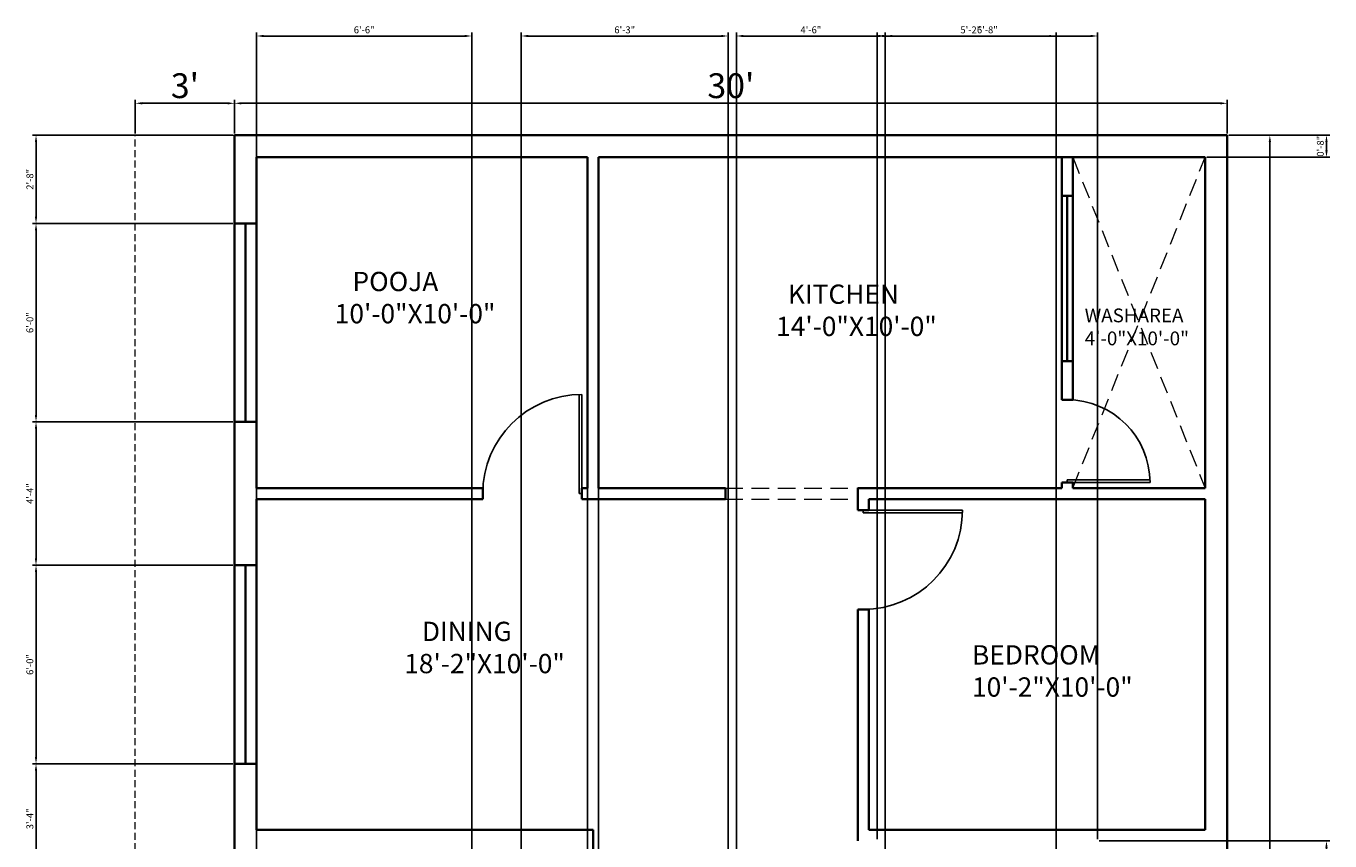
# Model space of a CAD drawing. Units: inches. Extents: x 1566 to 2546, y 1087 to 2705.
# Tile 26 of 27: x 1566 to 2039, y 2409 to 2705. Entities that reach past the tile are written whole.
import ezdxf

# ---------------------------------------------------------------- set-up
doc = ezdxf.new("R2010")
doc.units = ezdxf.units.IN
doc.linetypes.add('DASHED', pattern=[19.05, 12.7, -6.35])
for name, color, linetype, lineweight in [('A-ANNO-DIMS', 2, 'Continuous', 18), ('A-AREA-IDEN', 7, 'Continuous', 18), ('A-DOOR', 4, 'Continuous', 25), ('A-FLOR-OVHD', 8, 'DASHED', 18), ('A-WALL', 7, 'Continuous', 35)]:
    doc.layers.add(name, color=color, linetype=linetype, lineweight=lineweight)
doc.styles.get("Standard").update_dxf_attribs({"font": 'arial.ttf'})
doc.dimstyles.new('ISO-25', dxfattribs={"dimtxt": 2.5, "dimasz": 2.5, "dimexe": 1.25, "dimexo": 0.625, "dimtad": 1, "dimtxsty": 'Standard', "dimcen": 2.5, "dimadec": 0, "dimazin": 0, "dimtfac": 1, "dimtmove": 0, "dimatfit": 3, "dimfxl": 1, "dimarcsym": 0})

# ---------------------------------------------------------------- blocks, each defined once
blk = doc.blocks.new('d1')
for p, q in [((3297.32, 1596.93), (3297.32, 1632.93)), ((3298.32, 1596.93), (3298.32, 1632.93)), ((3297.32, 1596.93), (3298.32, 1596.93))]:
    blk.add_line(p, q)
at = {"ltscale": 0.3}
blk.add_arc((3297.32, 1596.93), 36, 0, 90, dxfattribs=at)
blk = doc.blocks.new('*D12')
at = {"layer": 'A-ANNO-DIMS', "color": 0, "lineweight": -2, "transparency": 16777216}
for p, q in [((2002.15, 2665.35), (2018.24, 2665.35)), ((2016.99, 2043.85), (2016.99, 2662.85)), ((2002.15, 2041.35), (2018.24, 2041.35))]:
    blk.add_line(p, q, dxfattribs=at)
at = {"layer": 'A-ANNO-DIMS', "color": 0, "transparency": 16777216}
for points in [[(2016.58, 2662.85), (2017.41, 2662.85), (2016.99, 2665.35)], [(2016.58, 2043.85), (2017.41, 2043.85), (2016.99, 2041.35)]]:
    blk.add_solid(points, dxfattribs=at)
at = {"layer": 'Defpoints', "color": 0, "transparency": 16777216}
for p in [(2001.53, 2665.35), (2016.99, 2665.35), (2001.53, 2041.35)]:
    blk.add_point(p, dxfattribs=at)
at = {"layer": 'A-ANNO-DIMS', "color": 0, "transparency": 16777216, "insert": (2011.77, 2353.35), "char_height": 9, "attachment_point": 5, "rotation": 90}
blk.add_mtext("52'", dxfattribs=at)
blk = doc.blocks.new('*D15')
at = {"layer": 'A-ANNO-DIMS', "color": 0, "lineweight": -2, "transparency": 16777216}
for p, q in [((1641.53, 2665.97), (1641.53, 2678.19)), ((1644.03, 2676.94), (1999.03, 2676.94)), ((2001.53, 2665.97), (2001.53, 2678.19))]:
    blk.add_line(p, q, dxfattribs=at)
at = {"layer": 'A-ANNO-DIMS', "color": 0, "transparency": 16777216}
for points in [[(1644.03, 2677.35), (1644.03, 2676.52), (1641.53, 2676.94)], [(1999.03, 2677.35), (1999.03, 2676.52), (2001.53, 2676.94)]]:
    blk.add_solid(points, dxfattribs=at)
at = {"layer": 'Defpoints', "color": 0, "transparency": 16777216}
for p in [(2001.53, 2676.94), (1641.53, 2665.35), (2001.53, 2665.35)]:
    blk.add_point(p, dxfattribs=at)
at = {"layer": 'A-ANNO-DIMS', "color": 0, "transparency": 16777216, "insert": (1821.53, 2682.16), "char_height": 9, "attachment_point": 5}
blk.add_mtext("30'", dxfattribs=at)
blk = doc.blocks.new('*D13')
at = {"layer": 'A-ANNO-DIMS', "color": 0, "lineweight": -2, "transparency": 16777216}
for p, q in [((1605.53, 2665.97), (1605.53, 2678.19)), ((1608.03, 2676.94), (1639.03, 2676.94)), ((1641.53, 2665.97), (1641.53, 2678.19))]:
    blk.add_line(p, q, dxfattribs=at)
at = {"layer": 'A-ANNO-DIMS', "color": 0, "transparency": 16777216}
for points in [[(1608.03, 2677.35), (1608.03, 2676.52), (1605.53, 2676.94)], [(1639.03, 2677.35), (1639.03, 2676.52), (1641.53, 2676.94)]]:
    blk.add_solid(points, dxfattribs=at)
at = {"layer": 'Defpoints', "color": 0, "transparency": 16777216}
for p in [(1641.53, 2676.94), (1605.53, 2665.35), (1641.53, 2665.35)]:
    blk.add_point(p, dxfattribs=at)
at = {"layer": 'A-ANNO-DIMS', "color": 0, "transparency": 16777216, "insert": (1623.53, 2682.16), "char_height": 9, "attachment_point": 5}
blk.add_mtext("3'", dxfattribs=at)
blk = doc.blocks.new('d2')
for p, q in [((3364.08, 1632.29), (3364.08, 1602.29)), ((3365.08, 1632.29), (3365.08, 1602.29)), ((3364.08, 1602.29), (3365.08, 1602.29))]:
    blk.add_line(p, q)
at = {"ltscale": 0.3}
blk.add_arc((3364.08, 1602.29), 30, 0, 90, dxfattribs=at)
blk = doc.blocks.new('*D69')
at = {"layer": 'A-ANNO-DIMS', "color": 0, "lineweight": -2, "transparency": 16777216}
for p, q in [((2002.15, 2665.35), (2038.78, 2665.35)), ((2037.53, 2662.85), (2037.53, 2659.85)), ((1994.15, 2657.35), (2038.78, 2657.35))]:
    blk.add_line(p, q, dxfattribs=at)
at = {"layer": 'A-ANNO-DIMS', "color": 0, "transparency": 16777216}
for points in [[(2037.11, 2662.85), (2037.95, 2662.85), (2037.53, 2665.35)], [(2037.11, 2659.85), (2037.95, 2659.85), (2037.53, 2657.35)]]:
    blk.add_solid(points, dxfattribs=at)
at = {"layer": 'Defpoints', "color": 0, "transparency": 16777216}
for p in [(2001.53, 2665.35), (1993.53, 2657.35), (2037.53, 2657.35)]:
    blk.add_point(p, dxfattribs=at)
at = {"layer": 'A-ANNO-DIMS', "color": 0, "transparency": 16777216, "insert": (2035.63, 2661.35), "char_height": 2.5, "attachment_point": 5, "rotation": 90}
blk.add_mtext('0\'-8"', dxfattribs=at)
blk = doc.blocks.new('*D70')
at = {"layer": 'A-ANNO-DIMS', "color": 0, "lineweight": -2, "transparency": 16777216}
for p, q in [((1769.53, 2656.72), (1769.53, 1974.1)), ((1773.53, 2656.72), (1773.53, 1974.1)), ((1767.03, 1975.35), (1764.53, 1975.35)), ((1769.53, 1975.35), (1773.53, 1975.35)), ((1776.03, 1975.35), (1786.43, 1975.35))]:
    blk.add_line(p, q, dxfattribs=at)
at = {"layer": 'A-ANNO-DIMS', "color": 0, "transparency": 16777216}
for points in [[(1767.03, 1975.76), (1767.03, 1974.93), (1769.53, 1975.35)], [(1776.03, 1975.76), (1776.03, 1974.93), (1773.53, 1975.35)]]:
    blk.add_solid(points, dxfattribs=at)
at = {"layer": 'Defpoints', "color": 0, "transparency": 16777216}
for p in [(1769.53, 2657.35), (1773.53, 2657.35), (1773.53, 1975.35)]:
    blk.add_point(p, dxfattribs=at)
at = {"layer": 'A-ANNO-DIMS', "color": 0, "transparency": 16777216, "insert": (1782.48, 1977.25), "char_height": 2.5, "attachment_point": 5}
blk.add_mtext('0\'-4"', dxfattribs=at)
blk = doc.blocks.new('*D71')
at = {"layer": 'A-ANNO-DIMS', "color": 0, "lineweight": -2, "transparency": 16777216}
for p, q in [((1640.9, 2665.35), (1568.28, 2665.35)), ((1569.53, 2662.85), (1569.53, 2635.85)), ((1640.9, 2633.35), (1568.28, 2633.35))]:
    blk.add_line(p, q, dxfattribs=at)
at = {"layer": 'A-ANNO-DIMS', "color": 0, "transparency": 16777216}
for points in [[(1569.11, 2662.85), (1569.95, 2662.85), (1569.53, 2665.35)], [(1569.11, 2635.85), (1569.95, 2635.85), (1569.53, 2633.35)]]:
    blk.add_solid(points, dxfattribs=at)
at = {"layer": 'Defpoints', "color": 0, "transparency": 16777216}
for p in [(1641.53, 2665.35), (1569.53, 2633.35), (1641.53, 2633.35)]:
    blk.add_point(p, dxfattribs=at)
at = {"layer": 'A-ANNO-DIMS', "color": 0, "transparency": 16777216, "insert": (1567.63, 2649.35), "char_height": 2.5, "attachment_point": 5, "rotation": 90}
blk.add_mtext('2\'-8"', dxfattribs=at)
blk = doc.blocks.new('*D72')
at = {"layer": 'A-ANNO-DIMS', "color": 0, "lineweight": -2, "transparency": 16777216}
for p, q in [((1640.9, 2633.35), (1568.28, 2633.35)), ((1569.53, 2630.85), (1569.53, 2563.85)), ((1640.9, 2561.35), (1568.28, 2561.35))]:
    blk.add_line(p, q, dxfattribs=at)
at = {"layer": 'A-ANNO-DIMS', "color": 0, "transparency": 16777216}
for points in [[(1569.11, 2630.85), (1569.95, 2630.85), (1569.53, 2633.35)], [(1569.11, 2563.85), (1569.95, 2563.85), (1569.53, 2561.35)]]:
    blk.add_solid(points, dxfattribs=at)
at = {"layer": 'Defpoints', "color": 0, "transparency": 16777216}
for p in [(1641.53, 2633.35), (1569.53, 2561.35), (1641.53, 2561.35)]:
    blk.add_point(p, dxfattribs=at)
at = {"layer": 'A-ANNO-DIMS', "color": 0, "transparency": 16777216, "insert": (1567.63, 2597.35), "char_height": 2.5, "attachment_point": 5, "rotation": 90}
blk.add_mtext('6\'-0"', dxfattribs=at)
blk = doc.blocks.new('*D73')
at = {"layer": 'A-ANNO-DIMS', "color": 0, "lineweight": -2, "transparency": 16777216}
for p, q in [((1640.9, 2561.35), (1568.28, 2561.35)), ((1569.53, 2558.85), (1569.53, 2511.85)), ((1640.9, 2509.35), (1568.28, 2509.35))]:
    blk.add_line(p, q, dxfattribs=at)
at = {"layer": 'A-ANNO-DIMS', "color": 0, "transparency": 16777216}
for points in [[(1569.11, 2558.85), (1569.95, 2558.85), (1569.53, 2561.35)], [(1569.11, 2511.85), (1569.95, 2511.85), (1569.53, 2509.35)]]:
    blk.add_solid(points, dxfattribs=at)
at = {"layer": 'Defpoints', "color": 0, "transparency": 16777216}
for p in [(1641.53, 2561.35), (1569.53, 2509.35), (1641.53, 2509.35)]:
    blk.add_point(p, dxfattribs=at)
at = {"layer": 'A-ANNO-DIMS', "color": 0, "transparency": 16777216, "insert": (1567.65, 2535.35), "char_height": 2.5, "attachment_point": 5, "rotation": 90}
blk.add_mtext('4\'-4"', dxfattribs=at)
blk = doc.blocks.new('*D74')
at = {"layer": 'A-ANNO-DIMS', "color": 0, "lineweight": -2, "transparency": 16777216}
for p, q in [((1640.9, 2509.35), (1568.28, 2509.35)), ((1569.53, 2506.85), (1569.53, 2439.85)), ((1640.9, 2437.35), (1568.28, 2437.35))]:
    blk.add_line(p, q, dxfattribs=at)
at = {"layer": 'A-ANNO-DIMS', "color": 0, "transparency": 16777216}
for points in [[(1569.11, 2506.85), (1569.95, 2506.85), (1569.53, 2509.35)], [(1569.11, 2439.85), (1569.95, 2439.85), (1569.53, 2437.35)]]:
    blk.add_solid(points, dxfattribs=at)
at = {"layer": 'Defpoints', "color": 0, "transparency": 16777216}
for p in [(1641.53, 2509.35), (1569.53, 2437.35), (1641.53, 2437.35)]:
    blk.add_point(p, dxfattribs=at)
at = {"layer": 'A-ANNO-DIMS', "color": 0, "transparency": 16777216, "insert": (1567.63, 2473.35), "char_height": 2.5, "attachment_point": 5, "rotation": 90}
blk.add_mtext('6\'-0"', dxfattribs=at)
blk = doc.blocks.new('*D75')
at = {"layer": 'A-ANNO-DIMS', "color": 0, "lineweight": -2, "transparency": 16777216}
for p, q in [((1640.9, 2437.35), (1568.28, 2437.35)), ((1569.53, 2434.85), (1569.53, 2399.85)), ((1640.9, 2397.35), (1568.28, 2397.35))]:
    blk.add_line(p, q, dxfattribs=at)
at = {"layer": 'A-ANNO-DIMS', "color": 0, "transparency": 16777216}
for points in [[(1569.11, 2434.85), (1569.95, 2434.85), (1569.53, 2437.35)], [(1569.11, 2399.85), (1569.95, 2399.85), (1569.53, 2397.35)]]:
    blk.add_solid(points, dxfattribs=at)
at = {"layer": 'Defpoints', "color": 0, "transparency": 16777216}
for p in [(1641.53, 2437.35), (1569.53, 2397.35), (1641.53, 2397.35)]:
    blk.add_point(p, dxfattribs=at)
at = {"layer": 'A-ANNO-DIMS', "color": 0, "transparency": 16777216, "insert": (1567.63, 2417.35), "char_height": 2.5, "attachment_point": 5, "rotation": 90}
blk.add_mtext('3\'-4"', dxfattribs=at)
blk = doc.blocks.new('*D79')
at = {"layer": 'A-ANNO-DIMS', "color": 0, "lineweight": -2, "transparency": 16777216}
for p, q in [((1649.53, 2165.97), (1649.53, 2702.6)), ((1652.03, 2701.35), (1725.03, 2701.35)), ((1727.53, 2165.97), (1727.53, 2702.6))]:
    blk.add_line(p, q, dxfattribs=at)
at = {"layer": 'A-ANNO-DIMS', "color": 0, "transparency": 16777216}
for points in [[(1652.03, 2701.76), (1652.03, 2700.93), (1649.53, 2701.35)], [(1725.03, 2701.76), (1725.03, 2700.93), (1727.53, 2701.35)]]:
    blk.add_solid(points, dxfattribs=at)
at = {"layer": 'Defpoints', "color": 0, "transparency": 16777216}
for p in [(1727.53, 2701.35), (1649.53, 2165.35), (1727.53, 2165.35)]:
    blk.add_point(p, dxfattribs=at)
at = {"layer": 'A-ANNO-DIMS', "color": 0, "transparency": 16777216, "insert": (1688.53, 2703.25), "char_height": 2.5, "attachment_point": 5}
blk.add_mtext('6\'-6"', dxfattribs=at)
blk = doc.blocks.new('*D81')
at = {"layer": 'A-ANNO-DIMS', "color": 0, "lineweight": -2, "transparency": 16777216}
for p, q in [((1823.53, 2098.97), (1823.53, 2702.6)), ((1826.03, 2701.35), (1875.03, 2701.35)), ((1877.53, 2098.97), (1877.53, 2702.6))]:
    blk.add_line(p, q, dxfattribs=at)
at = {"layer": 'A-ANNO-DIMS', "color": 0, "transparency": 16777216}
for points in [[(1826.03, 2701.76), (1826.03, 2700.93), (1823.53, 2701.35)], [(1875.03, 2701.76), (1875.03, 2700.93), (1877.53, 2701.35)]]:
    blk.add_solid(points, dxfattribs=at)
at = {"layer": 'Defpoints', "color": 0, "transparency": 16777216}
for p in [(1877.53, 2701.35), (1823.53, 2098.35), (1877.53, 2098.35)]:
    blk.add_point(p, dxfattribs=at)
at = {"layer": 'A-ANNO-DIMS', "color": 0, "transparency": 16777216, "insert": (1850.53, 2703.25), "char_height": 2.5, "attachment_point": 5}
blk.add_mtext('4\'-6"', dxfattribs=at)
blk = doc.blocks.new('*D82')
at = {"layer": 'A-ANNO-DIMS', "color": 0, "lineweight": -2, "transparency": 16777216}
for p, q in [((1877.53, 2098.97), (1877.53, 2702.6)), ((1880.03, 2701.35), (1937.03, 2701.35)), ((1939.53, 2098.97), (1939.53, 2702.6))]:
    blk.add_line(p, q, dxfattribs=at)
at = {"layer": 'A-ANNO-DIMS', "color": 0, "transparency": 16777216}
for points in [[(1880.03, 2701.76), (1880.03, 2700.93), (1877.53, 2701.35)], [(1937.03, 2701.76), (1937.03, 2700.93), (1939.53, 2701.35)]]:
    blk.add_solid(points, dxfattribs=at)
at = {"layer": 'Defpoints', "color": 0, "transparency": 16777216}
for p in [(1939.53, 2701.35), (1877.53, 2098.35), (1939.53, 2098.35)]:
    blk.add_point(p, dxfattribs=at)
at = {"layer": 'A-ANNO-DIMS', "color": 0, "transparency": 16777216, "insert": (1908.53, 2703.25), "char_height": 2.5, "attachment_point": 5}
blk.add_mtext('5\'-2"', dxfattribs=at)
blk = doc.blocks.new('*D83')
at = {"layer": 'A-ANNO-DIMS', "color": 0, "lineweight": -2, "transparency": 16777216}
for p, q in [((1874.53, 2409.97), (1874.53, 2702.6)), ((1877.03, 2701.35), (1952.03, 2701.35)), ((1954.53, 2409.97), (1954.53, 2702.6))]:
    blk.add_line(p, q, dxfattribs=at)
at = {"layer": 'A-ANNO-DIMS', "color": 0, "transparency": 16777216}
for points in [[(1877.03, 2701.76), (1877.03, 2700.93), (1874.53, 2701.35)], [(1952.03, 2701.76), (1952.03, 2700.93), (1954.53, 2701.35)]]:
    blk.add_solid(points, dxfattribs=at)
at = {"layer": 'Defpoints', "color": 0, "transparency": 16777216}
for p in [(1954.53, 2701.35), (1874.53, 2409.35), (1954.53, 2409.35)]:
    blk.add_point(p, dxfattribs=at)
at = {"layer": 'A-ANNO-DIMS', "color": 0, "transparency": 16777216, "insert": (1914.53, 2703.25), "char_height": 2.5, "attachment_point": 5}
blk.add_mtext('6\'-8"', dxfattribs=at)
blk = doc.blocks.new('*D84')
at = {"layer": 'A-ANNO-DIMS', "color": 0, "lineweight": -2, "transparency": 16777216}
for p, q in [((1955.15, 2409.35), (2038.78, 2409.35)), ((2037.53, 2406.85), (2037.53, 2372.85)), ((1955.15, 2370.35), (2038.78, 2370.35))]:
    blk.add_line(p, q, dxfattribs=at)
at = {"layer": 'A-ANNO-DIMS', "color": 0, "transparency": 16777216}
for points in [[(2037.11, 2406.85), (2037.95, 2406.85), (2037.53, 2409.35)], [(2037.11, 2372.85), (2037.95, 2372.85), (2037.53, 2370.35)]]:
    blk.add_solid(points, dxfattribs=at)
at = {"layer": 'Defpoints', "color": 0, "transparency": 16777216}
for p in [(1954.53, 2409.35), (1954.53, 2370.35), (2037.53, 2370.35)]:
    blk.add_point(p, dxfattribs=at)
at = {"layer": 'A-ANNO-DIMS', "color": 0, "transparency": 16777216, "insert": (2035.63, 2389.85), "char_height": 2.5, "attachment_point": 5, "rotation": 90}
blk.add_mtext('3\'-3"', dxfattribs=at)
blk = doc.blocks.new('*D86')
at = {"layer": 'A-ANNO-DIMS', "color": 0, "lineweight": -2, "transparency": 16777216}
for p, q in [((1745.53, 2041.97), (1745.53, 2702.6)), ((1748.03, 2701.35), (1818.03, 2701.35)), ((1820.53, 2041.97), (1820.53, 2702.6))]:
    blk.add_line(p, q, dxfattribs=at)
at = {"layer": 'A-ANNO-DIMS', "color": 0, "transparency": 16777216}
for points in [[(1748.03, 2701.76), (1748.03, 2700.93), (1745.53, 2701.35)], [(1818.03, 2701.76), (1818.03, 2700.93), (1820.53, 2701.35)]]:
    blk.add_solid(points, dxfattribs=at)
at = {"layer": 'Defpoints', "color": 0, "transparency": 16777216}
for p in [(1820.53, 2701.35), (1745.53, 2041.35), (1820.53, 2041.35)]:
    blk.add_point(p, dxfattribs=at)
at = {"layer": 'A-ANNO-DIMS', "color": 0, "transparency": 16777216, "insert": (1783.03, 2703.25), "char_height": 2.5, "attachment_point": 5}
blk.add_mtext('6\'-3"', dxfattribs=at)

msp = doc.modelspace()

# ---------------------------------------------------------------- linework, layer by layer
at = {"layer": 'A-FLOR-OVHD', "ltscale": 0.2}
for p, q in [((1605.53, 2017.35), (1605.53, 2665.35)), ((1605.53, 2665.35), (1641.53, 2665.35))]:
    msp.add_line(p, q, dxfattribs=at)
at = {"layer": 'A-FLOR-OVHD', "ltscale": 0.5}
for p, q in [((1945.53, 2657.35), (1993.53, 2537.35)), ((1945.53, 2537.35), (1993.53, 2657.35)), ((1819.53, 2537.35), (1867.53, 2537.35)), ((1819.53, 2533.35), (1867.53, 2533.35))]:
    msp.add_line(p, q, dxfattribs=at)
at = {"layer": 'A-WALL'}
for p, q in [((1641.53, 2665.35), (2001.53, 2665.35)), ((1641.53, 2041.35), (1641.53, 2665.35)), ((2001.53, 2665.35), (2001.53, 2041.35)), ((1649.53, 2657.35), (1769.53, 2657.35)), ((1649.53, 2537.35), (1649.53, 2657.35)), ((1769.53, 2537.35), (1769.53, 2657.35)), ((1773.53, 2657.35), (1993.53, 2657.35)), ((1773.53, 2537.35), (1773.53, 2657.35)), ((1941.53, 2569.35), (1941.53, 2657.35)), ((1945.53, 2569.28), (1945.53, 2657.35)), ((1993.53, 2657.35), (1993.53, 2537.35)), ((1941.53, 2643.34), (1945.53, 2643.34)), ((1943.53, 2643.34), (1943.53, 2583.34)), ((1641.53, 2633.35), (1649.53, 2633.35)), ((1645.53, 2633.35), (1645.53, 2561.35)), ((1941.53, 2583.34), (1945.53, 2583.34)), ((1941.53, 2569.35), (1945.53, 2569.35)), ((1649.53, 2561.35), (1641.53, 2561.35)), ((1941.53, 2537.35), (1941.53, 2539.35)), ((1941.53, 2539.35), (1945.53, 2539.35)), ((1941.53, 2537.35), (1941.53, 2539.35)), ((1945.53, 2537.35), (1945.53, 2539.35)), ((1945.53, 2537.35), (1945.53, 2539.35)), ((1649.53, 2537.35), (1731.53, 2537.35)), ((1731.53, 2533.35), (1731.53, 2537.35)), ((1767.53, 2537.35), (1769.53, 2537.35)), ((1767.53, 2533.35), (1767.53, 2537.35)), ((1773.53, 2537.35), (1819.53, 2537.35)), ((1819.53, 2537.35), (1819.53, 2533.35)), ((1867.53, 2537.35), (1941.53, 2537.35)), ((1867.53, 2537.35), (1867.53, 2529.35)), ((1945.53, 2537.35), (1993.53, 2537.35)), ((1649.53, 2533.35), (1731.53, 2533.35)), ((1649.53, 2413.35), (1649.53, 2533.35)), ((1767.53, 2533.35), (1819.53, 2533.35)), ((1871.53, 2533.35), (1993.53, 2533.35)), ((1871.53, 2533.35), (1871.53, 2529.35)), ((1993.53, 2533.35), (1993.53, 2413.35)), ((1867.53, 2529.35), (1871.53, 2529.35)), ((1641.53, 2509.35), (1649.53, 2509.35)), ((1645.53, 2509.35), (1645.53, 2437.35)), ((1867.53, 2493.35), (1871.53, 2493.35)), ((1867.53, 2493.35), (1867.53, 2409.35)), ((1871.53, 2493.35), (1871.53, 2413.35)), ((1649.53, 2437.35), (1641.53, 2437.35)), ((1649.53, 2413.35), (1771.53, 2413.35)), ((1771.53, 2387.35), (1771.53, 2413.35)), ((1871.53, 2413.35), (1993.53, 2413.35))]:
    msp.add_line(p, q, dxfattribs=at)

# ---------------------------------------------------------------- block references
at = {"layer": 'A-DOOR', "xscale": -1}
msp.add_blockref('d1', (5064.85, 938.42), dxfattribs=at)
at = {"layer": 'A-DOOR', "xscale": -1, "rotation": 270}
msp.add_blockref('d2', (341.24, -824.73), dxfattribs=at)
at = {"layer": 'A-DOOR', "rotation": 270}
msp.add_blockref('d1', (272.6, 5826.67), dxfattribs=at)

# ---------------------------------------------------------------- texts
at = {"layer": 'A-AREA-IDEN', "attachment_point": 1}
for s, insert, char_height in [('   POOJA\\P10\'-0"X10\'-0"', (1677.88, 2615.79), 7), ('  KITCHEN\\P14\'-0"X10\'-0"', (1837.94, 2611.19), 7), ('WASHAREA\\P4\'-0"X10\'-0"', (1949.85, 2602.49), 5), ('   DINING\\P18\'-2"X10\'-0"', (1703.07, 2488.86), 7), ('BEDROOM\\P10\'-2"X10\'-0"', (1908.98, 2480.35), 7)]:
    msp.add_mtext_dynamic_manual_height_columns(s, width=111.7553, gutter_width=12.5, heights=[0], dxfattribs=dict(at, insert=insert, char_height=char_height))

# ---------------------------------------------------------------- dimensions: what is measured, and where the dimension line sits
at = {"layer": 'A-ANNO-DIMS'}
for base, p1, p2, override, picture, middle in [((1727.53, 2701.35), (1649.53, 2165.35), (1727.53, 2165.35), {"dimdec": 1, "dimlfac": 1, "dimrnd": 0, "dimzin": 1, "dimdsep": 46, "dimlunit": 4, "dimfrac": 2}, '*D79', (1688.53, 2703.25)), ((1820.53, 2701.35), (1745.53, 2041.35), (1820.53, 2041.35), {"dimdec": 1, "dimlfac": 1, "dimrnd": 0, "dimzin": 1, "dimdsep": 46, "dimlunit": 4, "dimfrac": 2}, '*D86', (1783.03, 2703.25)), ((1877.53, 2701.35), (1823.53, 2098.35), (1877.53, 2098.35), {"dimdec": 1, "dimlfac": 1, "dimrnd": 0, "dimzin": 1, "dimdsep": 46, "dimlunit": 4, "dimfrac": 2}, '*D81', (1850.53, 2703.25)), ((1954.53, 2701.35), (1874.53, 2409.35), (1954.53, 2409.35), {"dimdec": 1, "dimlfac": 1, "dimrnd": 0, "dimzin": 1, "dimdsep": 46, "dimlunit": 4, "dimfrac": 2}, '*D83', (1914.53, 2703.25)), ((1939.53, 2701.35), (1877.53, 2098.35), (1939.53, 2098.35), {"dimdec": 1, "dimlfac": 1, "dimrnd": 0, "dimzin": 1, "dimdsep": 46, "dimlunit": 4, "dimfrac": 2}, '*D82', (1908.53, 2703.25)), ((1641.53, 2676.94), (1605.53, 2665.35), (1641.53, 2665.35), {"dimtxt": 9, "dimdec": 1, "dimlunit": 3, "dimclrd": 0, "dimclre": 0, "dimclrt": 0, "dimtdec": 1}, '*D13', (1623.53, 2682.16)), ((2001.53, 2676.94), (1641.53, 2665.35), (2001.53, 2665.35), {"dimtxt": 9, "dimdec": 1, "dimlunit": 3, "dimclrd": 0, "dimclre": 0, "dimclrt": 0, "dimtdec": 1}, '*D15', (1821.53, 2682.16)), ((1773.53, 1975.35), (1769.53, 2657.35), (1773.53, 2657.35), {"dimdec": 1, "dimlfac": 1, "dimrnd": 0, "dimzin": 1, "dimdsep": 46, "dimlunit": 4, "dimfrac": 2}, '*D70', (1782.48, 1977.25))]:
    dim = msp.add_linear_dim(base=base, p1=p1, p2=p2, dimstyle='ISO-25', override=override, dxfattribs=at)
    dim.commit()
    dim.dimension.update_dxf_attribs({"geometry": picture, "text_midpoint": middle})
for base, p1, p2, override, picture, middle in [((1569.53, 2633.35), (1641.53, 2665.35), (1641.53, 2633.35), {"dimdec": 1, "dimlfac": 1, "dimrnd": 0, "dimzin": 1, "dimdsep": 46, "dimlunit": 4, "dimfrac": 2}, '*D71', (1567.63, 2649.35)), ((2037.53, 2657.35), (2001.53, 2665.35), (1993.53, 2657.35), {"dimdec": 1, "dimlfac": 1, "dimrnd": 0, "dimzin": 1, "dimdsep": 46, "dimlunit": 4, "dimfrac": 2}, '*D69', (2035.63, 2661.35)), ((2016.99, 2665.35), (2001.53, 2041.35), (2001.53, 2665.35), {"dimtxt": 9, "dimdec": 1, "dimlunit": 3, "dimclrd": 0, "dimclre": 0, "dimclrt": 0, "dimtdec": 1}, '*D12', (2011.77, 2353.35)), ((1569.53, 2561.35), (1641.53, 2633.35), (1641.53, 2561.35), {"dimdec": 1, "dimlfac": 1, "dimrnd": 0, "dimzin": 1, "dimdsep": 46, "dimlunit": 4, "dimfrac": 2}, '*D72', (1567.63, 2597.35)), ((1569.53, 2509.35), (1641.53, 2561.35), (1641.53, 2509.35), {"dimdec": 1, "dimlfac": 1, "dimrnd": 0, "dimzin": 1, "dimdsep": 46, "dimlunit": 4, "dimfrac": 2}, '*D73', (1567.65, 2535.35)), ((1569.53, 2437.35), (1641.53, 2509.35), (1641.53, 2437.35), {"dimdec": 1, "dimlfac": 1, "dimrnd": 0, "dimzin": 1, "dimdsep": 46, "dimlunit": 4, "dimfrac": 2}, '*D74', (1567.63, 2473.35)), ((1569.53, 2397.35), (1641.53, 2437.35), (1641.53, 2397.35), {"dimdec": 1, "dimlfac": 1, "dimrnd": 0, "dimzin": 1, "dimdsep": 46, "dimlunit": 4, "dimfrac": 2}, '*D75', (1567.63, 2417.35)), ((2037.53, 2370.35), (1954.53, 2409.35), (1954.53, 2370.35), {"dimdec": 1, "dimlfac": 1, "dimrnd": 0, "dimzin": 1, "dimdsep": 46, "dimlunit": 4, "dimfrac": 2}, '*D84', (2035.63, 2389.85))]:
    dim = msp.add_linear_dim(base=base, p1=p1, p2=p2, angle=90, dimstyle='ISO-25', override=override, dxfattribs=at)
    dim.commit()
    dim.dimension.update_dxf_attribs({"geometry": picture, "text_midpoint": middle})

doc.saveas('drawing.dxf')
